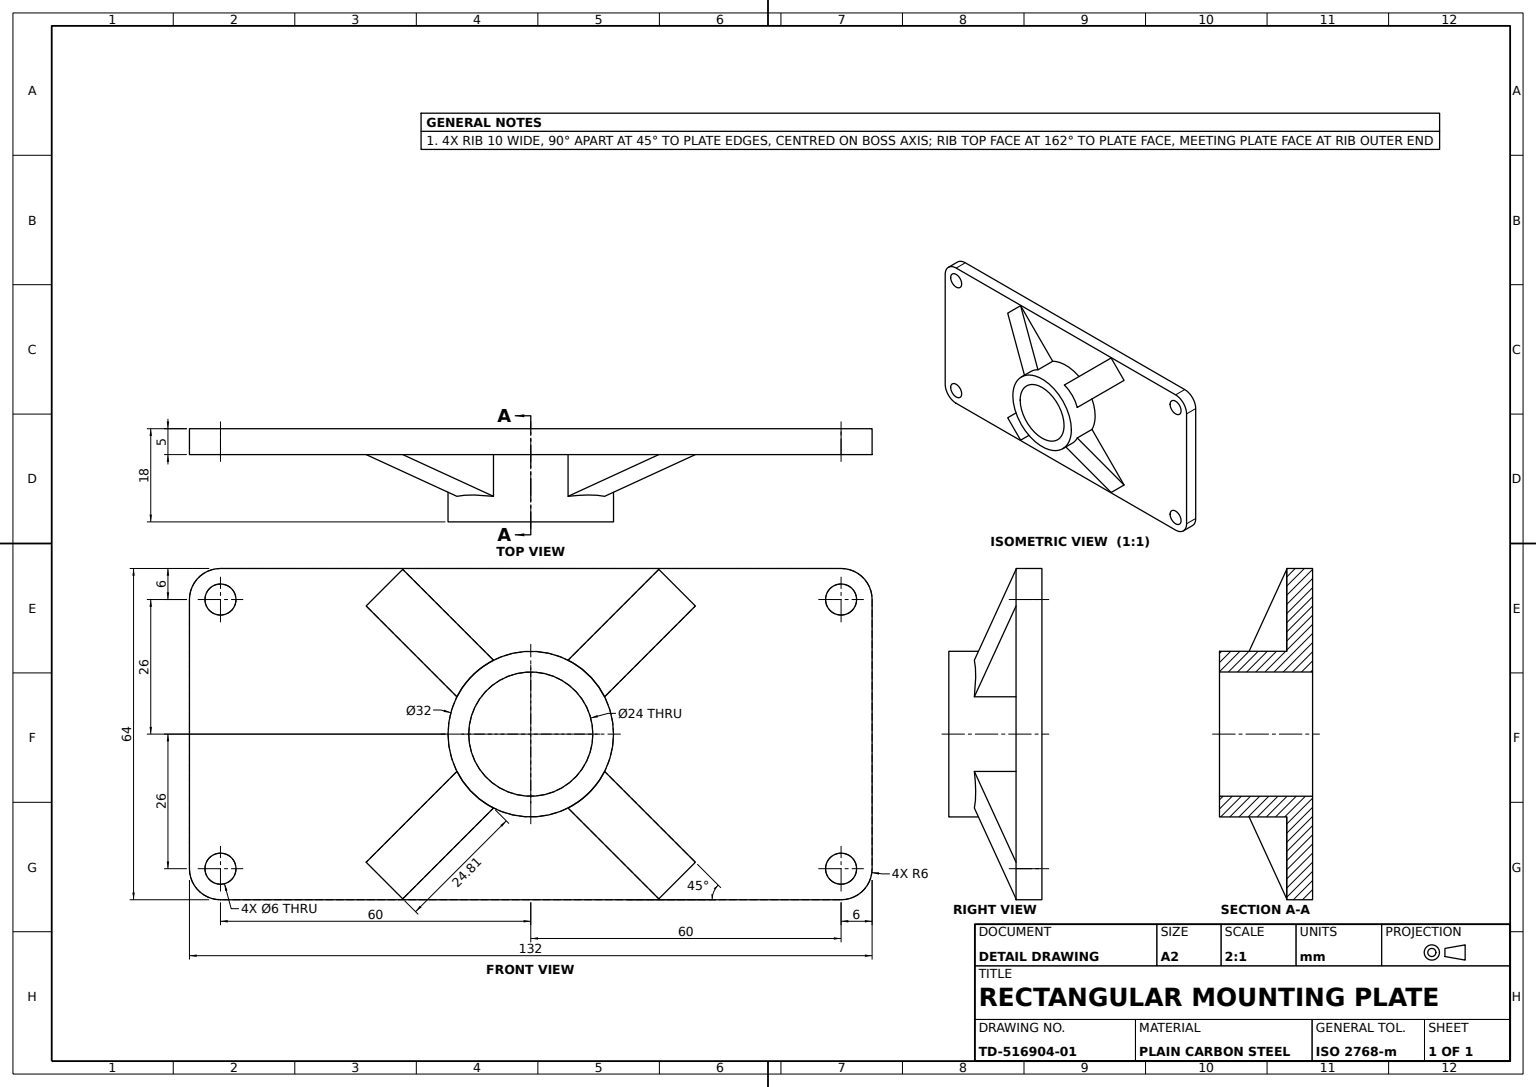
SolidWorks part; units mm, degrees
material "Plain Carbon Steel"
ref_plane "Front Plane" through (0, 0, 0) normal (0, 0, 1) x (1, 0, 0)
ref_plane "Top Plane" through (0, 0, 0) normal (0, 1, 0) x (1, 0, 0)
ref_plane "Right Plane" through (0, 0, 0) normal (1, 0, 0) x (0, 0, -1)
sketch "Plate Profile" plane through (0, 0, 0) normal (0, 0, 1) x (1, 0, 0)
  line L1 (-60, -32) -> (60, -32)
  line L2 (-66, -26) -> (-66, 26)
  line L3 (-60, 32) -> (60, 32)
  line L4 (66, -26) -> (66, 26)
  line L5 (-66, -32) -> (66, 32) construction
  line L6 (-66, 32) -> (66, -32) construction
  arc A0 (-66, -26) -> (-60, -32) centre (-60, -26) ccw
  arc A1 (60, -32) -> (66, -26) centre (60, -26) ccw
  arc A2 (60, 32) -> (66, 26) centre (60, 26) cw
  arc A3 (-66, 26) -> (-60, 32) centre (-60, 26) cw
  circle A4 centre (-60, 26) radius 3
  circle A5 centre (60, 26) radius 3
  circle A6 centre (60, -26) radius 3
  circle A7 centre (-60, -26) radius 3
  circle A8 centre (0, 0) radius 12
  circle A9 centre (0, 0) radius 16 construction
  point P0 (0, 0)
  dimension "D3" = 6
  dimension "D4" = 6
  dimension "D5" = 32
  dimension "D6" = 24
  dimension "D1" = 132
  dimension "D2" = 64
extrude "Base Plate 132x64x5" add sketch "Plate Profile" along normal blind 5
sketch "Hub Profile" plane through (0, 0, 5) normal (0, 0, 1) x (1, 0, 0)
  circle A0 centre (0, 0) radius 12 construction
  circle A1 centre (0, 0) radius 16 construction
  circle A2 centre (0, 0) radius 12
  circle A3 centre (0, 0) radius 16
extrude "Hub Boss" add sketch "Hub Profile" along normal blind 13
ref_plane "Rib Plane" through (0, 0, 0) normal (-0.7071, 0.7071, 0) x (0.7071, 0.7071, 0)
sketch "Rib Profile" plane through (0, 0, 0) normal (-0.7071, 0.7071, 0) x (0.7071, 0.7071, 0)
  line L0 (0, -18) -> (-42.7975, -4.0942)
  line L1 (-16, -18) -> (16, -18) construction
  line L4 (-65.0538, -5) -> (19.799, -5) construction
  dimension "D1" = 45
  dimension "D2" = 162
rib "Hub Rib 10mm" sketch "Rib Profile" sketch "Rib Profile" thickness 10 extrusion direction parallel to sketch draft on no parameters "D1"=10
pattern_circular "Rib Pattern 4x" count 4 over 360 about axis through (0, 0, 0) along (0, 0, 1) of "Hub Rib 10mm"
